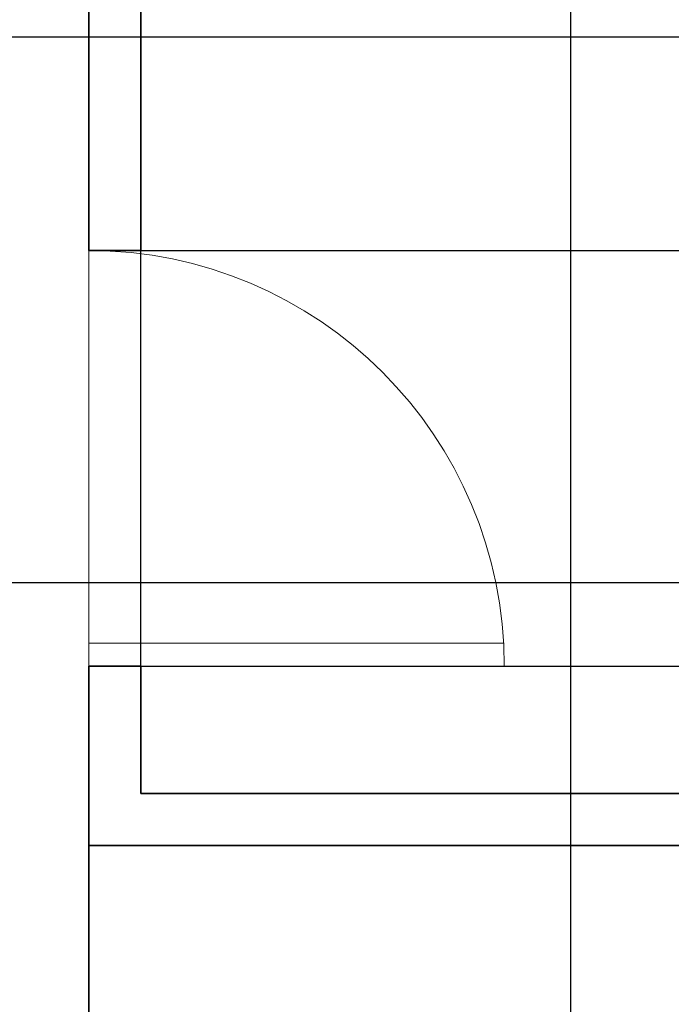
# Model space of a CAD drawing. Units: inches. Extents: x -26 to 385, y 12 to 697.
# Tile 3 of 13: x 136 to 192, y 130 to 215. Entities that reach past the tile are written whole.
import ezdxf

# ---------------------------------------------------------------- set-up
doc = ezdxf.new("R2010")
doc.units = ezdxf.units.IN
doc.header["$MEASUREMENT"] = 0
for name, color, linetype, lineweight in [('A-ANNO-DIMS', 4, 'Continuous', 18), ('A-DOOR', 30, 'Continuous', 20), ('A-WALL', 40, 'Continuous', 35)]:
    doc.layers.add(name, color=color, linetype=linetype, lineweight=lineweight)
doc.styles.get("Standard").update_dxf_attribs({"font": 'italic8.shx'})
doc.dimstyles.get("Standard").update_dxf_attribs({"dimtxt": 8, "dimasz": 0.18, "dimexe": 0.18, "dimexo": 0.0625, "dimgap": 0.09, "dimtad": 0, "dimtih": 1, "dimtoh": 1, "dimdec": 4, "dimzin": 0, "dimdsep": 46, "dimlunit": 3, "dimtxsty": 'Standard', "dimcen": 0.09, "dimclrd": 2, "dimclre": 3, "dimclrt": 6, "dimadec": 0, "dimazin": 0, "dimtfac": 1, "dimtdec": 4, "dimtofl": 0, "dimtmove": 0, "dimatfit": 3, "dimfxl": 1, "dimtolj": 1, "dimtzin": 0, "dimarcsym": 0})

# ---------------------------------------------------------------- blocks, each defined once
blk = doc.blocks.new('*D28')
at = {"layer": 'A-ANNO-DIMS', "color": 3, "lineweight": -2, "transparency": 16777216}
for p, q in [((141.692, 194.903), (355.559, 194.903)), ((141.692, 158.903), (355.559, 158.903))]:
    blk.add_line(p, q, dxfattribs=at)
at = {"layer": 'A-ANNO-DIMS', "color": 2, "lineweight": -2, "transparency": 16777216}
for p, q in [((355.379, 194.723), (355.379, 181.755)), ((355.379, 159.083), (355.379, 172.052))]:
    blk.add_line(p, q, dxfattribs=at)
at = {"layer": 'A-ANNO-DIMS', "color": 2, "transparency": 16777216}
for points in [[(355.349, 194.723), (355.409, 194.723), (355.379, 194.903)], [(355.349, 159.083), (355.409, 159.083), (355.379, 158.903)]]:
    blk.add_solid(points, dxfattribs=at)
at = {"layer": 'Defpoints', "color": 0, "transparency": 16777216}
for p in [(141.629, 194.903), (355.379, 194.903), (141.629, 158.903)]:
    blk.add_point(p, dxfattribs=at)
at = {"layer": 'A-ANNO-DIMS', "color": 6, "transparency": 16777216, "insert": (355.379, 176.903), "char_height": 8, "attachment_point": 5}
blk.add_mtext('\\A1;3\'-0"', dxfattribs=at)
blk = doc.blocks.new('*D32')
at = {"layer": 'A-ANNO-DIMS', "color": 3, "lineweight": -2, "transparency": 16777216}
for p, q in [((239.825, 213.385), (-5.301, 213.385)), ((239.825, 166.141), (-5.301, 166.141))]:
    blk.add_line(p, q, dxfattribs=at)
at = {"layer": 'A-ANNO-DIMS', "color": 2, "lineweight": -2, "transparency": 16777216}
for p, q in [((-5.121, 213.205), (-5.121, 194.615)), ((-5.121, 166.321), (-5.121, 184.911))]:
    blk.add_line(p, q, dxfattribs=at)
at = {"layer": 'A-ANNO-DIMS', "color": 2, "transparency": 16777216}
for points in [[(-5.151, 213.205), (-5.091, 213.205), (-5.121, 213.385)], [(-5.151, 166.321), (-5.091, 166.321), (-5.121, 166.141)]]:
    blk.add_solid(points, dxfattribs=at)
at = {"layer": 'Defpoints', "color": 0, "transparency": 16777216}
for p in [(-5.121, 213.385), (239.888, 213.385), (239.888, 166.141)]:
    blk.add_point(p, dxfattribs=at)
at = {"layer": 'A-ANNO-DIMS', "color": 6, "transparency": 16777216, "insert": (-5.121, 189.763), "char_height": 8, "attachment_point": 5}
blk.add_mtext('\\A1;3\'-11"', dxfattribs=at)
blk = doc.blocks.new('*D33')
at = {"layer": 'A-ANNO-DIMS', "color": 3, "lineweight": -2, "transparency": 16777216}
for p, q in [((58.468, 279.817), (58.468, 23.949)), ((97.847, 279.817), (97.847, 23.949))]:
    blk.add_line(p, q, dxfattribs=at)
at = {"layer": 'A-ANNO-DIMS', "color": 2, "lineweight": -2, "transparency": 16777216}
for p, q in [((58.648, 24.129), (97.667, 24.129)), ((97.847, 24.129), (98.027, 24.129))]:
    blk.add_line(p, q, dxfattribs=at)
at = {"layer": 'A-ANNO-DIMS', "color": 2, "transparency": 16777216}
for points in [[(58.648, 24.159), (58.648, 24.099), (58.468, 24.129)], [(97.667, 24.159), (97.667, 24.099), (97.847, 24.129)]]:
    blk.add_solid(points, dxfattribs=at)
at = {"layer": 'Defpoints', "color": 0, "transparency": 16777216}
for p in [(58.468, 279.879), (97.847, 279.879), (97.847, 24.129)]:
    blk.add_point(p, dxfattribs=at)
at = {"layer": 'A-ANNO-DIMS', "color": 6, "transparency": 16777216, "insert": (131.259, 24.129), "char_height": 8, "attachment_point": 5}
blk.add_mtext('\\A1;3\'-3 1/2"', dxfattribs=at)
blk = doc.blocks.new('*D36')
at = {"layer": 'A-ANNO-DIMS', "color": 3, "lineweight": -2, "transparency": 16777216}
for p, q in [((146.129, 147.942), (146.129, 684.809)), ((193.598, 147.942), (193.598, 684.809))]:
    blk.add_line(p, q, dxfattribs=at)
at = {"layer": 'A-ANNO-DIMS', "color": 2, "lineweight": -2, "transparency": 16777216}
for p, q in [((146.309, 684.629), (193.418, 684.629)), ((193.598, 684.629), (193.778, 684.629))]:
    blk.add_line(p, q, dxfattribs=at)
at = {"layer": 'A-ANNO-DIMS', "color": 2, "transparency": 16777216}
for points in [[(146.309, 684.659), (146.309, 684.599), (146.129, 684.629)], [(193.418, 684.659), (193.418, 684.599), (193.598, 684.629)]]:
    blk.add_solid(points, dxfattribs=at)
at = {"layer": 'Defpoints', "color": 0, "transparency": 16777216}
for p in [(193.598, 684.629), (146.129, 147.879), (193.598, 147.879)]:
    blk.add_point(p, dxfattribs=at)
at = {"layer": 'A-ANNO-DIMS', "color": 6, "transparency": 16777216, "insert": (228.344, 684.629), "char_height": 8, "attachment_point": 5}
blk.add_mtext('\\A1;3\'-11 1/2"', dxfattribs=at)
blk = doc.blocks.new('*D39')
at = {"layer": 'A-ANNO-DIMS', "color": 3, "lineweight": -2, "transparency": 16777216}
for p, q in [((183.359, 597.317), (183.359, 23.949)), ((213.359, 597.317), (213.359, 23.949))]:
    blk.add_line(p, q, dxfattribs=at)
at = {"layer": 'A-ANNO-DIMS', "color": 2, "lineweight": -2, "transparency": 16777216}
for p, q in [((183.539, 24.129), (213.179, 24.129)), ((213.359, 24.129), (213.539, 24.129))]:
    blk.add_line(p, q, dxfattribs=at)
at = {"layer": 'A-ANNO-DIMS', "color": 2, "transparency": 16777216}
for points in [[(183.539, 24.159), (183.539, 24.099), (183.359, 24.129)], [(213.179, 24.159), (213.179, 24.099), (213.359, 24.129)]]:
    blk.add_solid(points, dxfattribs=at)
at = {"layer": 'Defpoints', "color": 0, "transparency": 16777216}
for p in [(183.359, 597.379), (213.359, 597.379), (213.359, 24.129)]:
    blk.add_point(p, dxfattribs=at)
at = {"layer": 'A-ANNO-DIMS', "color": 6, "transparency": 16777216, "insert": (231.533, 24.129), "char_height": 8, "attachment_point": 5}
blk.add_mtext('\\A1;2\'-6"', dxfattribs=at)
blk = doc.blocks.new('*D55')
at = {"layer": 'A-ANNO-DIMS', "color": 3, "lineweight": -2, "transparency": 16777216}
for p, q in [((146.192, 158.903), (355.559, 158.903)), ((146.192, 147.879), (355.559, 147.879))]:
    blk.add_line(p, q, dxfattribs=at)
at = {"layer": 'A-ANNO-DIMS', "color": 2, "lineweight": -2, "transparency": 16777216}
for p, q in [((355.379, 158.723), (355.379, 158.243)), ((355.379, 148.059), (355.379, 148.539))]:
    blk.add_line(p, q, dxfattribs=at)
at = {"layer": 'A-ANNO-DIMS', "color": 2, "transparency": 16777216}
for points in [[(355.349, 158.723), (355.409, 158.723), (355.379, 158.903)], [(355.349, 148.059), (355.409, 148.059), (355.379, 147.879)]]:
    blk.add_solid(points, dxfattribs=at)
at = {"layer": 'Defpoints', "color": 0, "transparency": 16777216}
for p in [(146.129, 158.903), (355.379, 158.903), (146.129, 147.879)]:
    blk.add_point(p, dxfattribs=at)
at = {"layer": 'A-ANNO-DIMS', "color": 6, "transparency": 16777216, "insert": (355.379, 153.391), "char_height": 8, "attachment_point": 5}
blk.add_mtext('\\A1;0\'-11"', dxfattribs=at)

msp = doc.modelspace()

# ---------------------------------------------------------------- linework, layer by layer
at = {"layer": 'A-DOOR'}
for p, q in [((141.62932, 194.90341), (141.62932, 158.90341)), ((141.62932, 160.90341), (177.62932, 160.90341)), ((141.62932, 158.90341), (177.62932, 158.90341))]:
    msp.add_line(p, q, dxfattribs=at)
msp.add_arc((141.62932, 158.90341), 36, 0, 90, dxfattribs=at)
at = {"layer": 'A-WALL'}
for p, q in [((146.12932, 332.37909), (146.12932, 194.90341)), ((141.62932, 275.37909), (141.62932, 194.90341)), ((146.12932, 194.90341), (141.62932, 194.90341)), ((146.12932, 158.90341), (141.62932, 158.90341)), ((141.62932, 158.90341), (141.62932, 54.37909)), ((146.12932, 158.90341), (146.12932, 147.87909)), ((320.62932, 147.87909), (146.12932, 147.87909)), ((320.62932, 143.37909), (141.62932, 143.37909))]:
    msp.add_line(p, q, dxfattribs=at)

# ---------------------------------------------------------------- dimensions: what is measured, and where the dimension line sits
at = {"layer": 'A-ANNO-DIMS'}
for base, p1, p2, picture, middle in [((193.59818, 684.62909), (146.12932, 147.87909), (193.59818, 147.87909), '*D36', (228.34437, 684.62909)), ((213.35855, 24.12909), (183.35855, 597.37909), (213.35855, 597.37909), '*D39', (231.53331, 24.12909)), ((97.84659, 24.12909), (58.46784, 279.87909), (97.84659, 279.87909), '*D33', (131.25945, 24.12909))]:
    dim = msp.add_linear_dim(base=base, p1=p1, p2=p2, dimstyle='Standard', override={"dimdec": 1, "dimlfac": 1, "dimrnd": 0, "dimzin": 1, "dimdsep": 46, "dimlunit": 4, "dimfrac": 2}, dxfattribs=at)
    dim.commit()
    dim.dimension.update_dxf_attribs({"geometry": picture, "text_midpoint": middle})
for base, p1, p2, picture, middle in [((-5.12068, 213.38513), (239.88756, 166.14113), (239.88756, 213.38513), '*D32', (-5.12068, 189.76313)), ((355.37932, 194.90341), (141.62932, 158.90341), (141.62932, 194.90341), '*D28', (355.37932, 176.90341)), ((355.37932, 158.90341), (146.12932, 147.87909), (146.12932, 158.90341), '*D55', (355.37932, 153.39125))]:
    dim = msp.add_linear_dim(base=base, p1=p1, p2=p2, angle=90, dimstyle='Standard', override={"dimdec": 1, "dimlfac": 1, "dimrnd": 0, "dimzin": 1, "dimdsep": 46, "dimlunit": 4, "dimfrac": 2}, dxfattribs=at)
    dim.commit()
    dim.dimension.update_dxf_attribs({"geometry": picture, "text_midpoint": middle})

doc.saveas('drawing.dxf')
